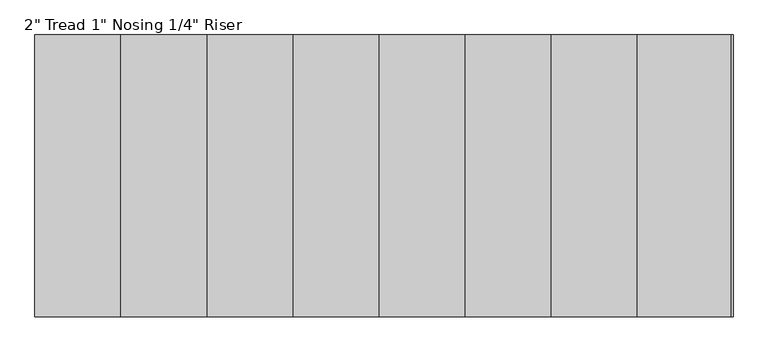
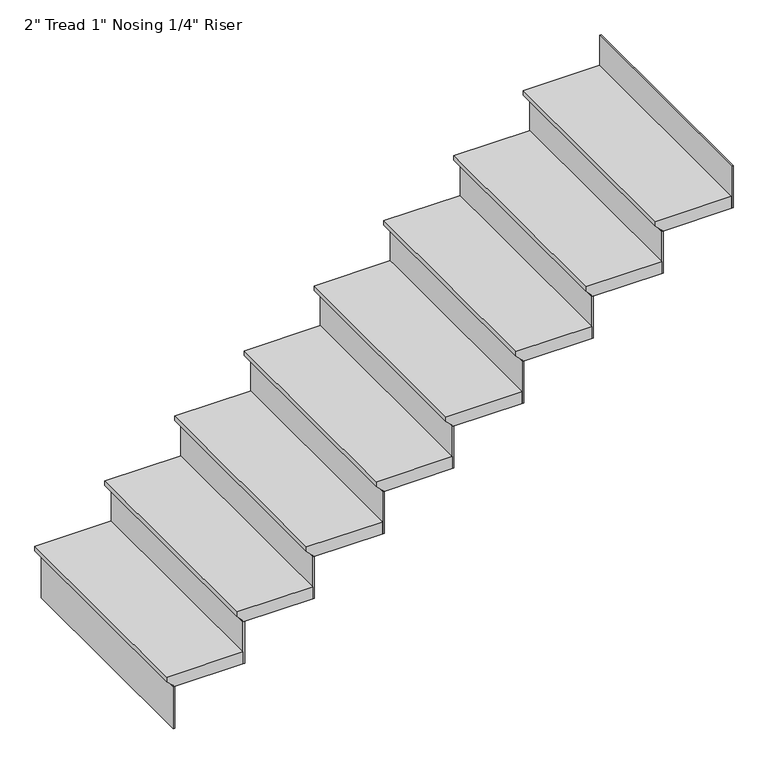
"""IFC4 building model written with IfcOpenShell, lengths in millimetres: stair flight geometry."""

from ifc_helpers import new_model, si_unit, frame, origin, place, context, project, spatial, polyline, outline, extrude, source, transform, mapped, element, save


def stair_flight_3143a382(model_context):
    return source(origin(), model_context, "Body", "SweptSolid", [
        extrude(outline(polyline([(1778.0, -6244.1591614), (1778.0, -6548.9591614), (1758.95, -6548.9591614), (1733.55, -6523.5591614), (1727.2, -6523.5591614), (1727.2, -6244.1591614), (1778.0, -6244.1591614)])), frame((0.0, 402.4325188, 0.0), z_axis=(0.0, 1.0, 0.0), x_axis=(0.0, 0.0, 1.0)), (0.0, 0.0, 1.0), 914.4),
        extrude(outline(polyline([(-6517.2091614, 402.4325188), (-6523.5591614, 402.4325188), (-6523.5591614, 1316.8325188), (-6517.2091614, 1316.8325188), (-6517.2091614, 402.4325188)])), frame((0.0, 0.0, 1549.4), z_axis=(0.0, 0.0, 1.0), x_axis=(1.0, 0.0, 0.0)), (0.0, 0.0, 1.0), 177.8),
        extrude(outline(polyline([(-6237.8091614, 402.4325188), (-6244.1591614, 402.4325188), (-6244.1591614, 1316.8325188), (-6237.8091614, 1316.8325188), (-6237.8091614, 402.4325188)])), frame((0.0, 0.0, 1727.2), z_axis=(0.0, 0.0, 1.0), x_axis=(1.0, 0.0, 0.0)), (0.0, 0.0, 1.0), 177.8),
        extrude(outline(polyline([(1955.8, -5964.7591614), (1955.8, -6269.5591614), (1936.75, -6269.5591614), (1911.35, -6244.1591614), (1905.0, -6244.1591614), (1905.0, -5964.7591614), (1955.8, -5964.7591614)])), frame((0.0, 402.4325188, 0.0), z_axis=(0.0, 1.0, 0.0), x_axis=(0.0, 0.0, 1.0)), (0.0, 0.0, 1.0), 914.4),
        extrude(outline(polyline([(-5958.4091614, 402.4325188), (-5964.7591614, 402.4325188), (-5964.7591614, 1316.8325188), (-5958.4091614, 1316.8325188), (-5958.4091614, 402.4325188)])), frame((0.0, 0.0, 1905.0), z_axis=(0.0, 0.0, 1.0), x_axis=(1.0, 0.0, 0.0)), (0.0, 0.0, 1.0), 177.8),
        extrude(outline(polyline([(2133.6, -5685.3591614), (2133.6, -5990.1591614), (2114.55, -5990.1591614), (2089.15, -5964.7591614), (2082.8, -5964.7591614), (2082.8, -5685.3591614), (2133.6, -5685.3591614)])), frame((0.0, 402.4325188, 0.0), z_axis=(0.0, 1.0, 0.0), x_axis=(0.0, 0.0, 1.0)), (0.0, 0.0, 1.0), 914.4),
        extrude(outline(polyline([(-5679.0091614, 402.4325188), (-5685.3591614, 402.4325188), (-5685.3591614, 1316.8325188), (-5679.0091614, 1316.8325188), (-5679.0091614, 402.4325188)])), frame((0.0, 0.0, 2082.8), z_axis=(0.0, 0.0, 1.0), x_axis=(1.0, 0.0, 0.0)), (0.0, 0.0, 1.0), 177.8),
        extrude(outline(polyline([(2311.4, -5405.9591614), (2311.4, -5710.7591614), (2292.35, -5710.7591614), (2266.95, -5685.3591614), (2260.6, -5685.3591614), (2260.6, -5405.9591614), (2311.4, -5405.9591614)])), frame((0.0, 402.4325188, 0.0), z_axis=(0.0, 1.0, 0.0), x_axis=(0.0, 0.0, 1.0)), (0.0, 0.0, 1.0), 914.4),
        extrude(outline(polyline([(-5399.6091614, 402.4325188), (-5405.9591614, 402.4325188), (-5405.9591614, 1316.8325188), (-5399.6091614, 1316.8325188), (-5399.6091614, 402.4325188)])), frame((0.0, 0.0, 2260.6), z_axis=(0.0, 0.0, 1.0), x_axis=(1.0, 0.0, 0.0)), (0.0, 0.0, 1.0), 177.8),
        extrude(outline(polyline([(2489.2, -5126.5591614), (2489.2, -5431.3591614), (2470.15, -5431.3591614), (2444.75, -5405.9591614), (2438.4, -5405.9591614), (2438.4, -5126.5591614), (2489.2, -5126.5591614)])), frame((0.0, 402.4325188, 0.0), z_axis=(0.0, 1.0, 0.0), x_axis=(0.0, 0.0, 1.0)), (0.0, 0.0, 1.0), 914.4),
        extrude(outline(polyline([(-5120.2091614, 402.4325188), (-5126.5591614, 402.4325188), (-5126.5591614, 1316.8325188), (-5120.2091614, 1316.8325188), (-5120.2091614, 402.4325188)])), frame((0.0, 0.0, 2438.4), z_axis=(0.0, 0.0, 1.0), x_axis=(1.0, 0.0, 0.0)), (0.0, 0.0, 1.0), 177.8),
        extrude(outline(polyline([(2667.0, -4847.1591614), (2667.0, -5151.9591614), (2647.95, -5151.9591614), (2622.55, -5126.5591614), (2616.2, -5126.5591614), (2616.2, -4847.1591614), (2667.0, -4847.1591614)])), frame((0.0, 402.4325188, 0.0), z_axis=(0.0, 1.0, 0.0), x_axis=(0.0, 0.0, 1.0)), (0.0, 0.0, 1.0), 914.4),
        extrude(outline(polyline([(-4840.8091614, 402.4325188), (-4847.1591614, 402.4325188), (-4847.1591614, 1316.8325188), (-4840.8091614, 1316.8325188), (-4840.8091614, 402.4325188)])), frame((0.0, 0.0, 2616.2), z_axis=(0.0, 0.0, 1.0), x_axis=(1.0, 0.0, 0.0)), (0.0, 0.0, 1.0), 177.8),
        extrude(outline(polyline([(2844.8, -4567.7591614), (2844.8, -4872.5591614), (2825.75, -4872.5591614), (2800.35, -4847.1591614), (2794.0, -4847.1591614), (2794.0, -4567.7591614), (2844.8, -4567.7591614)])), frame((0.0, 402.4325188, 0.0), z_axis=(0.0, 1.0, 0.0), x_axis=(0.0, 0.0, 1.0)), (0.0, 0.0, 1.0), 914.4),
        extrude(outline(polyline([(-4561.4091614, 402.4325188), (-4567.7591614, 402.4325188), (-4567.7591614, 1316.8325188), (-4561.4091614, 1316.8325188), (-4561.4091614, 402.4325188)])), frame((0.0, 0.0, 2794.0), z_axis=(0.0, 0.0, 1.0), x_axis=(1.0, 0.0, 0.0)), (0.0, 0.0, 1.0), 177.8),
        extrude(outline(polyline([(-4282.0091614, 402.4325188), (-4288.3591614, 402.4325188), (-4288.3591614, 1316.8325188), (-4282.0091614, 1316.8325188), (-4282.0091614, 402.4325188)])), frame((0.0, 0.0, 2971.8), z_axis=(0.0, 0.0, 1.0), x_axis=(1.0, 0.0, 0.0)), (0.0, 0.0, 1.0), 177.8),
        extrude(outline(polyline([(3022.6, -4288.3591614), (3022.6, -4593.1591614), (3003.55, -4593.1591614), (2978.15, -4567.7591614), (2971.8, -4567.7591614), (2971.8, -4288.3591614), (3022.6, -4288.3591614)])), frame((0.0, 402.4325188, 0.0), z_axis=(0.0, 1.0, 0.0), x_axis=(0.0, 0.0, 1.0)), (0.0, 0.0, 1.0), 914.4),
    ])


if __name__ == "__main__":
    model = new_model("IFC4")
    model_context = context("Model", 3, world=origin())
    ifc_project = project(units=[si_unit("LENGTHUNIT", "METRE", prefix="MILLI")], contexts=[model_context])
    site = spatial("IfcSite", under=ifc_project)
    building = spatial("IfcBuilding", under=site)
    placement = place(None, origin())
    stair_flight_shape = stair_flight_3143a382(model_context)
    element("IfcStairFlight", 1, ObjectType="2\" Tread 1\" Nosing 1/4\" Riser", at=placement, inside=building, context=model_context, shape_type="MappedRepresentation", body=[
        mapped(stair_flight_shape, transform((0.0, 0.0, 0.0), x_axis=(1.0, 0.0, 0.0), y_axis=(0.0, 1.0, 0.0), z_axis=(0.0, 0.0, 1.0))),
    ])
    save(model, "model.ifc")
